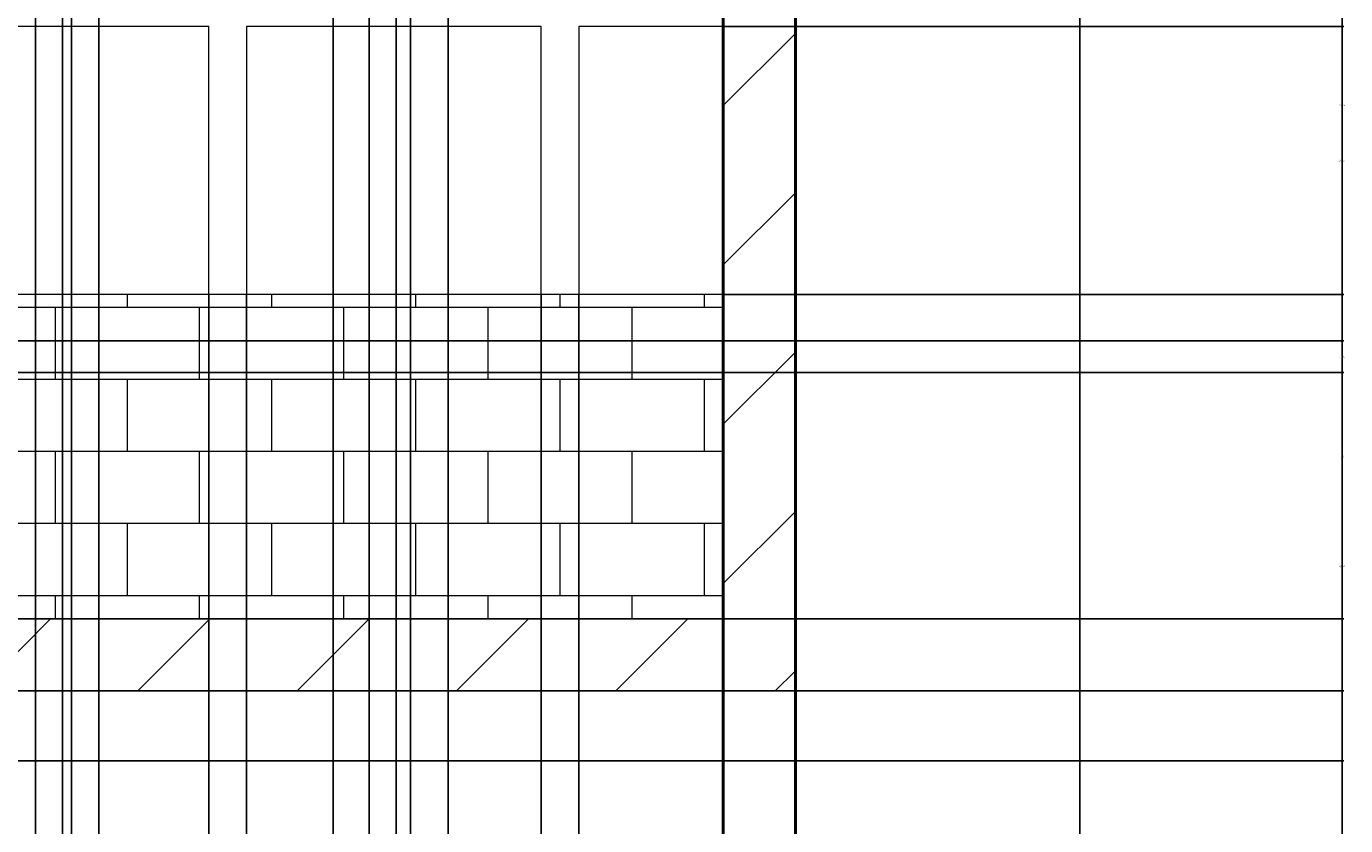
# Model space of a CAD drawing. Units: inches. Extents: x -14 to 375, y -86 to 549.
# Tile 9 of 12: x 228 to 375, y 248 to 336. Entities that reach past the tile are written whole.
import ezdxf

# ---------------------------------------------------------------- set-up
doc = ezdxf.new("R2010")
doc.units = ezdxf.units.IN
doc.header["$MEASUREMENT"] = 0
for name, color, linetype, lineweight in [('A-ANNO-DIMS', 2, 'Continuous', 18), ('A-ELEV', 7, 'Continuous', 25), ('A-ELEV-PATT', 8, 'Continuous', 13), ('A-ELEV-RAIL', 8, 'Continuous', 18)]:
    doc.layers.add(name, color=color, linetype=linetype, lineweight=lineweight)
doc.styles.get("Standard").update_dxf_attribs({"font": 'arial.ttf'})
doc.dimstyles.get("Standard").update_dxf_attribs({"dimtxt": 0.18, "dimasz": 0.18, "dimexe": 0.18, "dimexo": 0.0625, "dimgap": 0.09, "dimtad": 0, "dimtih": 1, "dimtoh": 1, "dimdec": 4, "dimzin": 0, "dimdsep": 46, "dimtxsty": 'Standard', "dimcen": 0.09, "dimadec": 0, "dimazin": 0, "dimtfac": 1, "dimtdec": 4, "dimtofl": 0, "dimtmove": 0, "dimatfit": 3, "dimfxl": 1, "dimtolj": 1, "dimtzin": 0, "dimarcsym": 0})

# ---------------------------------------------------------------- blocks, each defined once
blk = doc.blocks.new('*D10')
at = {"layer": 'A-ANNO-DIMS', "color": 0, "lineweight": -2, "transparency": 16777216}
for p, q in [((301.52, 485.96), (374.54, 485.96)), ((374.36, 485.78), (374.36, 225.61)), ((374.36, -34.93), (374.36, 225.24)), ((345.33, -35.11), (374.54, -35.11))]:
    blk.add_line(p, q, dxfattribs=at)
at = {"layer": 'A-ANNO-DIMS', "color": 0, "transparency": 16777216}
for points in [[(374.33, 485.78), (374.39, 485.78), (374.36, 485.96)], [(374.33, -34.93), (374.39, -34.93), (374.36, -35.11)]]:
    blk.add_solid(points, dxfattribs=at)
at = {"layer": 'Defpoints', "color": 0, "transparency": 16777216}
for p in [(301.46, 485.96), (374.36, 485.96), (345.26, -35.11)]:
    blk.add_point(p, dxfattribs=at)
at = {"layer": 'A-ANNO-DIMS', "color": 0, "transparency": 16777216, "insert": (374.36, 225.42), "char_height": 0.18, "attachment_point": 5}
blk.add_mtext('\\A1;521.1', dxfattribs=at)
blk = doc.blocks.new('*D33')
at = {"layer": 'A-ANNO-DIMS', "color": 0, "lineweight": -2, "transparency": 16777216}
for p, q in [((107.76, 254.96), (374.54, 254.96)), ((374.36, 254.78), (374.36, 250.64)), ((374.36, 246.14), (374.36, 250.28)), ((107.76, 245.96), (374.54, 245.96))]:
    blk.add_line(p, q, dxfattribs=at)
at = {"layer": 'A-ANNO-DIMS', "color": 0, "transparency": 16777216}
for points in [[(374.33, 254.78), (374.39, 254.78), (374.36, 254.96)], [(374.33, 246.14), (374.39, 246.14), (374.36, 245.96)]]:
    blk.add_solid(points, dxfattribs=at)
at = {"layer": 'Defpoints', "color": 0, "transparency": 16777216}
for p in [(107.7, 254.96), (374.36, 254.96), (107.7, 245.96)]:
    blk.add_point(p, dxfattribs=at)
at = {"layer": 'A-ANNO-DIMS', "color": 0, "transparency": 16777216, "insert": (374.36, 250.46), "char_height": 0.18, "attachment_point": 5}
blk.add_mtext('\\A1;9', dxfattribs=at)
blk = doc.blocks.new('*D34')
at = {"layer": 'A-ANNO-DIMS', "color": 0, "lineweight": -2, "transparency": 16777216}
for p, q in [((107.64, 298.04), (374.54, 298.04)), ((374.36, 297.86), (374.36, 276.68)), ((374.36, 255.14), (374.36, 276.32)), ((107.76, 254.96), (374.54, 254.96))]:
    blk.add_line(p, q, dxfattribs=at)
at = {"layer": 'A-ANNO-DIMS', "color": 0, "transparency": 16777216}
for points in [[(374.33, 297.86), (374.39, 297.86), (374.36, 298.04)], [(374.33, 255.14), (374.39, 255.14), (374.36, 254.96)]]:
    blk.add_solid(points, dxfattribs=at)
at = {"layer": 'Defpoints', "color": 0, "transparency": 16777216}
for p in [(107.58, 298.04), (374.36, 298.04), (107.7, 254.96)]:
    blk.add_point(p, dxfattribs=at)
at = {"layer": 'A-ANNO-DIMS', "color": 0, "transparency": 16777216, "insert": (374.36, 276.5), "char_height": 0.18, "attachment_point": 5}
blk.add_mtext('\\A1;43.08', dxfattribs=at)
blk = doc.blocks.new('*D35')
at = {"layer": 'A-ANNO-DIMS', "color": 0, "lineweight": -2, "transparency": 16777216}
for p, q in [((107.64, 301.54), (374.54, 301.54)), ((374.36, 301.36), (374.36, 299.97)), ((374.36, 298.22), (374.36, 299.6)), ((107.64, 298.04), (374.54, 298.04))]:
    blk.add_line(p, q, dxfattribs=at)
at = {"layer": 'A-ANNO-DIMS', "color": 0, "transparency": 16777216}
for points in [[(374.33, 301.36), (374.39, 301.36), (374.36, 301.54)], [(374.33, 298.22), (374.39, 298.22), (374.36, 298.04)]]:
    blk.add_solid(points, dxfattribs=at)
at = {"layer": 'Defpoints', "color": 0, "transparency": 16777216}
for p in [(107.58, 301.54), (374.36, 301.54), (107.58, 298.04)]:
    blk.add_point(p, dxfattribs=at)
at = {"layer": 'A-ANNO-DIMS', "color": 0, "transparency": 16777216, "insert": (374.36, 299.79), "char_height": 0.18, "attachment_point": 5}
blk.add_mtext('\\A1;3.501', dxfattribs=at)
blk = doc.blocks.new('*D36')
at = {"layer": 'A-ANNO-DIMS', "color": 0, "lineweight": -2, "transparency": 16777216}
for p, q in [((107.56, 353.96), (374.54, 353.96)), ((374.36, 353.78), (374.36, 327.93)), ((374.36, 301.72), (374.36, 327.57)), ((107.64, 301.54), (374.54, 301.54))]:
    blk.add_line(p, q, dxfattribs=at)
at = {"layer": 'A-ANNO-DIMS', "color": 0, "transparency": 16777216}
for points in [[(374.33, 353.78), (374.39, 353.78), (374.36, 353.96)], [(374.33, 301.72), (374.39, 301.72), (374.36, 301.54)]]:
    blk.add_solid(points, dxfattribs=at)
at = {"layer": 'Defpoints', "color": 0, "transparency": 16777216}
for p in [(107.5, 353.96), (374.36, 353.96), (107.58, 301.54)]:
    blk.add_point(p, dxfattribs=at)
at = {"layer": 'A-ANNO-DIMS', "color": 0, "transparency": 16777216, "insert": (374.36, 327.75), "char_height": 0.18, "attachment_point": 5}
blk.add_mtext('\\A1;52.42', dxfattribs=at)
blk = doc.blocks.new('*D43')
at = {"layer": 'A-ANNO-DIMS', "color": 0, "lineweight": -2, "transparency": 16777216}
for p, q in [((142.23, 270.64), (142.23, -64.39)), ((305.63, 270.64), (305.63, -64.39)), ((142.41, -64.21), (223.55, -64.21)), ((305.45, -64.21), (224.32, -64.21))]:
    blk.add_line(p, q, dxfattribs=at)
at = {"layer": 'A-ANNO-DIMS', "color": 0, "transparency": 16777216}
for points in [[(142.41, -64.18), (142.41, -64.24), (142.23, -64.21)], [(305.45, -64.18), (305.45, -64.24), (305.63, -64.21)]]:
    blk.add_solid(points, dxfattribs=at)
at = {"layer": 'Defpoints', "color": 0, "transparency": 16777216}
for p in [(142.23, 270.71), (305.63, 270.71), (305.63, -64.21)]:
    blk.add_point(p, dxfattribs=at)
at = {"layer": 'A-ANNO-DIMS', "color": 0, "transparency": 16777216, "insert": (223.93, -64.21), "char_height": 0.18, "attachment_point": 5}
blk.add_mtext('\\A1;163.4', dxfattribs=at)
blk = doc.blocks.new('*D44')
at = {"layer": 'A-ANNO-DIMS', "color": 0, "lineweight": -2, "transparency": 16777216}
for p, q in [((305.63, 270.64), (305.63, -64.39)), ((313.63, 262.64), (313.63, -64.39)), ((305.81, -64.21), (309.48, -64.21)), ((313.45, -64.21), (309.78, -64.21))]:
    blk.add_line(p, q, dxfattribs=at)
at = {"layer": 'A-ANNO-DIMS', "color": 0, "transparency": 16777216}
for points in [[(305.81, -64.18), (305.81, -64.24), (305.63, -64.21)], [(313.45, -64.18), (313.45, -64.24), (313.63, -64.21)]]:
    blk.add_solid(points, dxfattribs=at)
at = {"layer": 'Defpoints', "color": 0, "transparency": 16777216}
for p in [(305.63, 270.71), (313.63, 262.71), (313.63, -64.21)]:
    blk.add_point(p, dxfattribs=at)
at = {"layer": 'A-ANNO-DIMS', "color": 0, "transparency": 16777216, "insert": (309.63, -64.21), "char_height": 0.18, "attachment_point": 5}
blk.add_mtext('\\A1;8', dxfattribs=at)
blk = doc.blocks.new('*D49')
at = {"layer": 'A-ANNO-DIMS', "color": 0, "lineweight": -2, "transparency": 16777216}
for p, q in [((215.95, 306.64), (215.95, -64.39)), ((248.64, 306.64), (248.64, -64.39)), ((216.13, -64.21), (231.9, -64.21)), ((248.46, -64.21), (232.69, -64.21))]:
    blk.add_line(p, q, dxfattribs=at)
at = {"layer": 'A-ANNO-DIMS', "color": 0, "transparency": 16777216}
for points in [[(216.13, -64.18), (216.13, -64.24), (215.95, -64.21)], [(248.46, -64.18), (248.46, -64.24), (248.64, -64.21)]]:
    blk.add_solid(points, dxfattribs=at)
at = {"layer": 'Defpoints', "color": 0, "transparency": 16777216}
for p in [(215.95, 306.71), (248.64, 306.71), (248.64, -64.21)]:
    blk.add_point(p, dxfattribs=at)
at = {"layer": 'A-ANNO-DIMS', "color": 0, "transparency": 16777216, "insert": (232.29, -64.21), "char_height": 0.18, "attachment_point": 5}
blk.add_mtext('\\A1;32.69', dxfattribs=at)
blk = doc.blocks.new('*D50')
at = {"layer": 'A-ANNO-DIMS', "color": 0, "lineweight": -2, "transparency": 16777216}
for p, q in [((248.64, 306.64), (248.64, -64.39)), ((252.81, 306.64), (252.81, -64.39)), ((248.82, -64.21), (250.39, -64.21)), ((252.63, -64.21), (251.05, -64.21))]:
    blk.add_line(p, q, dxfattribs=at)
at = {"layer": 'A-ANNO-DIMS', "color": 0, "transparency": 16777216}
for points in [[(248.82, -64.18), (248.82, -64.24), (248.64, -64.21)], [(252.63, -64.18), (252.63, -64.24), (252.81, -64.21)]]:
    blk.add_solid(points, dxfattribs=at)
at = {"layer": 'Defpoints', "color": 0, "transparency": 16777216}
for p in [(248.64, 306.71), (252.81, 306.71), (252.81, -64.21)]:
    blk.add_point(p, dxfattribs=at)
at = {"layer": 'A-ANNO-DIMS', "color": 0, "transparency": 16777216, "insert": (250.72, -64.21), "char_height": 0.18, "attachment_point": 5}
blk.add_mtext('\\A1;4.17', dxfattribs=at)
blk = doc.blocks.new('*D51')
at = {"layer": 'A-ANNO-DIMS', "color": 0, "lineweight": -2, "transparency": 16777216}
for p, q in [((252.81, 306.64), (252.81, -64.39)), ((285.5, 306.64), (285.5, -64.39)), ((252.99, -64.21), (268.76, -64.21)), ((285.32, -64.21), (269.54, -64.21))]:
    blk.add_line(p, q, dxfattribs=at)
at = {"layer": 'A-ANNO-DIMS', "color": 0, "transparency": 16777216}
for points in [[(252.99, -64.18), (252.99, -64.24), (252.81, -64.21)], [(285.32, -64.18), (285.32, -64.24), (285.5, -64.21)]]:
    blk.add_solid(points, dxfattribs=at)
at = {"layer": 'Defpoints', "color": 0, "transparency": 16777216}
for p in [(252.81, 306.71), (285.5, 306.71), (285.5, -64.21)]:
    blk.add_point(p, dxfattribs=at)
at = {"layer": 'A-ANNO-DIMS', "color": 0, "transparency": 16777216, "insert": (269.15, -64.21), "char_height": 0.18, "attachment_point": 5}
blk.add_mtext('\\A1;32.69', dxfattribs=at)
blk = doc.blocks.new('*D52')
at = {"layer": 'A-ANNO-DIMS', "color": 0, "lineweight": -2, "transparency": 16777216}
for p, q in [((285.5, 306.64), (285.5, -64.39)), ((289.66, 306.64), (289.66, -64.39)), ((285.68, -64.21), (287.25, -64.21)), ((289.48, -64.21), (287.91, -64.21))]:
    blk.add_line(p, q, dxfattribs=at)
at = {"layer": 'A-ANNO-DIMS', "color": 0, "transparency": 16777216}
for points in [[(285.68, -64.18), (285.68, -64.24), (285.5, -64.21)], [(289.48, -64.18), (289.48, -64.24), (289.66, -64.21)]]:
    blk.add_solid(points, dxfattribs=at)
at = {"layer": 'Defpoints', "color": 0, "transparency": 16777216}
for p in [(285.5, 306.71), (289.66, 306.71), (289.66, -64.21)]:
    blk.add_point(p, dxfattribs=at)
at = {"layer": 'A-ANNO-DIMS', "color": 0, "transparency": 16777216, "insert": (287.58, -64.21), "char_height": 0.18, "attachment_point": 5}
blk.add_mtext('\\A1;4.17', dxfattribs=at)
blk = doc.blocks.new('*D57')
at = {"layer": 'A-ANNO-DIMS', "color": 0, "lineweight": -2, "transparency": 16777216}
for p, q in [((229.41, 340.38), (229.41, -64.39)), ((232.41, 340.38), (232.41, -64.39)), ((229.59, -64.21), (230.76, -64.21)), ((232.23, -64.21), (231.06, -64.21))]:
    blk.add_line(p, q, dxfattribs=at)
at = {"layer": 'A-ANNO-DIMS', "color": 0, "transparency": 16777216}
for points in [[(229.59, -64.18), (229.59, -64.24), (229.41, -64.21)], [(232.23, -64.18), (232.23, -64.24), (232.41, -64.21)]]:
    blk.add_solid(points, dxfattribs=at)
at = {"layer": 'Defpoints', "color": 0, "transparency": 16777216}
for p in [(229.41, 340.44), (232.41, 340.44), (232.41, -64.21)]:
    blk.add_point(p, dxfattribs=at)
at = {"layer": 'A-ANNO-DIMS', "color": 0, "transparency": 16777216, "insert": (230.91, -64.21), "char_height": 0.18, "attachment_point": 5}
blk.add_mtext('\\A1;3', dxfattribs=at)
blk = doc.blocks.new('*D58')
at = {"layer": 'A-ANNO-DIMS', "color": 0, "lineweight": -2, "transparency": 16777216}
for p, q in [((232.41, 340.38), (232.41, -64.39)), ((236.41, 340.38), (236.41, -64.39)), ((232.59, -64.21), (234.26, -64.21)), ((236.23, -64.21), (234.56, -64.21))]:
    blk.add_line(p, q, dxfattribs=at)
at = {"layer": 'A-ANNO-DIMS', "color": 0, "transparency": 16777216}
for points in [[(232.59, -64.18), (232.59, -64.24), (232.41, -64.21)], [(236.23, -64.18), (236.23, -64.24), (236.41, -64.21)]]:
    blk.add_solid(points, dxfattribs=at)
at = {"layer": 'Defpoints', "color": 0, "transparency": 16777216}
for p in [(232.41, 340.44), (236.41, 340.44), (236.41, -64.21)]:
    blk.add_point(p, dxfattribs=at)
at = {"layer": 'A-ANNO-DIMS', "color": 0, "transparency": 16777216, "insert": (234.41, -64.21), "char_height": 0.18, "attachment_point": 5}
blk.add_mtext('\\A1;4', dxfattribs=at)
blk = doc.blocks.new('*D59')
at = {"layer": 'A-ANNO-DIMS', "color": 0, "lineweight": -2, "transparency": 16777216}
for p, q in [((236.41, 340.38), (236.41, -64.39)), ((262.41, 340.38), (262.41, -64.39)), ((236.59, -64.21), (249.19, -64.21)), ((262.23, -64.21), (249.63, -64.21))]:
    blk.add_line(p, q, dxfattribs=at)
at = {"layer": 'A-ANNO-DIMS', "color": 0, "transparency": 16777216}
for points in [[(236.59, -64.18), (236.59, -64.24), (236.41, -64.21)], [(262.23, -64.18), (262.23, -64.24), (262.41, -64.21)]]:
    blk.add_solid(points, dxfattribs=at)
at = {"layer": 'Defpoints', "color": 0, "transparency": 16777216}
for p in [(236.41, 340.44), (262.41, 340.44), (262.41, -64.21)]:
    blk.add_point(p, dxfattribs=at)
at = {"layer": 'A-ANNO-DIMS', "color": 0, "transparency": 16777216, "insert": (249.41, -64.21), "char_height": 0.18, "attachment_point": 5}
blk.add_mtext('\\A1;26', dxfattribs=at)
blk = doc.blocks.new('*D60')
at = {"layer": 'A-ANNO-DIMS', "color": 0, "lineweight": -2, "transparency": 16777216}
for p, q in [((262.41, 340.38), (262.41, -64.39)), ((266.41, 340.38), (266.41, -64.39)), ((262.59, -64.21), (264.26, -64.21)), ((266.23, -64.21), (264.56, -64.21))]:
    blk.add_line(p, q, dxfattribs=at)
at = {"layer": 'A-ANNO-DIMS', "color": 0, "transparency": 16777216}
for points in [[(262.59, -64.18), (262.59, -64.24), (262.41, -64.21)], [(266.23, -64.18), (266.23, -64.24), (266.41, -64.21)]]:
    blk.add_solid(points, dxfattribs=at)
at = {"layer": 'Defpoints', "color": 0, "transparency": 16777216}
for p in [(262.41, 340.44), (266.41, 340.44), (266.41, -64.21)]:
    blk.add_point(p, dxfattribs=at)
at = {"layer": 'A-ANNO-DIMS', "color": 0, "transparency": 16777216, "insert": (264.41, -64.21), "char_height": 0.18, "attachment_point": 5}
blk.add_mtext('\\A1;4', dxfattribs=at)
blk = doc.blocks.new('*D61')
at = {"layer": 'A-ANNO-DIMS', "color": 0, "lineweight": -2, "transparency": 16777216}
for p, q in [((266.41, 340.38), (266.41, -64.39)), ((269.41, 340.38), (269.41, -64.39)), ((266.59, -64.21), (267.76, -64.21)), ((269.23, -64.21), (268.06, -64.21))]:
    blk.add_line(p, q, dxfattribs=at)
at = {"layer": 'A-ANNO-DIMS', "color": 0, "transparency": 16777216}
for points in [[(266.59, -64.18), (266.59, -64.24), (266.41, -64.21)], [(269.23, -64.18), (269.23, -64.24), (269.41, -64.21)]]:
    blk.add_solid(points, dxfattribs=at)
at = {"layer": 'Defpoints', "color": 0, "transparency": 16777216}
for p in [(266.41, 340.44), (269.41, 340.44), (269.41, -64.21)]:
    blk.add_point(p, dxfattribs=at)
at = {"layer": 'A-ANNO-DIMS', "color": 0, "transparency": 16777216, "insert": (267.91, -64.21), "char_height": 0.18, "attachment_point": 5}
blk.add_mtext('\\A1;3', dxfattribs=at)
blk = doc.blocks.new('*D62')
at = {"layer": 'A-ANNO-DIMS', "color": 0, "lineweight": -2, "transparency": 16777216}
for p, q in [((305.69, 270.71), (374.54, 270.71)), ((374.36, 270.53), (374.36, 266.89)), ((374.36, 262.89), (374.36, 266.53)), ((313.69, 262.71), (374.54, 262.71))]:
    blk.add_line(p, q, dxfattribs=at)
at = {"layer": 'A-ANNO-DIMS', "color": 0, "transparency": 16777216}
for points in [[(374.33, 270.53), (374.39, 270.53), (374.36, 270.71)], [(374.33, 262.89), (374.39, 262.89), (374.36, 262.71)]]:
    blk.add_solid(points, dxfattribs=at)
at = {"layer": 'Defpoints', "color": 0, "transparency": 16777216}
for p in [(305.63, 270.71), (374.36, 270.71), (313.63, 262.71)]:
    blk.add_point(p, dxfattribs=at)
at = {"layer": 'A-ANNO-DIMS', "color": 0, "transparency": 16777216, "insert": (374.36, 266.71), "char_height": 0.18, "attachment_point": 5}
blk.add_mtext('\\A1;8', dxfattribs=at)
blk = doc.blocks.new('*D63')
at = {"layer": 'A-ANNO-DIMS', "color": 0, "lineweight": -2, "transparency": 16777216}
for p, q in [((305.69, 306.71), (374.54, 306.71)), ((374.36, 306.53), (374.36, 288.89)), ((374.36, 270.89), (374.36, 288.53)), ((305.69, 270.71), (374.54, 270.71))]:
    blk.add_line(p, q, dxfattribs=at)
at = {"layer": 'A-ANNO-DIMS', "color": 0, "transparency": 16777216}
for points in [[(374.33, 306.53), (374.39, 306.53), (374.36, 306.71)], [(374.33, 270.89), (374.39, 270.89), (374.36, 270.71)]]:
    blk.add_solid(points, dxfattribs=at)
at = {"layer": 'Defpoints', "color": 0, "transparency": 16777216}
for p in [(305.63, 306.71), (374.36, 306.71), (305.63, 270.71)]:
    blk.add_point(p, dxfattribs=at)
at = {"layer": 'A-ANNO-DIMS', "color": 0, "transparency": 16777216, "insert": (374.36, 288.71), "char_height": 0.18, "attachment_point": 5}
blk.add_mtext('\\A1;36', dxfattribs=at)
blk = doc.blocks.new('*D64')
at = {"layer": 'A-ANNO-DIMS', "color": 0, "lineweight": -2, "transparency": 16777216}
for p, q in [((305.69, 336.44), (374.54, 336.44)), ((374.36, 336.26), (374.36, 321.76)), ((374.36, 306.89), (374.36, 321.39)), ((305.69, 306.71), (374.54, 306.71))]:
    blk.add_line(p, q, dxfattribs=at)
at = {"layer": 'A-ANNO-DIMS', "color": 0, "transparency": 16777216}
for points in [[(374.33, 336.26), (374.39, 336.26), (374.36, 336.44)], [(374.33, 306.89), (374.39, 306.89), (374.36, 306.71)]]:
    blk.add_solid(points, dxfattribs=at)
at = {"layer": 'Defpoints', "color": 0, "transparency": 16777216}
for p in [(305.63, 336.44), (374.36, 336.44), (305.63, 306.71)]:
    blk.add_point(p, dxfattribs=at)
at = {"layer": 'A-ANNO-DIMS', "color": 0, "transparency": 16777216, "insert": (374.36, 321.57), "char_height": 0.18, "attachment_point": 5}
blk.add_mtext('\\A1;29.735', dxfattribs=at)
blk = doc.blocks.new('*D72')
at = {"layer": 'A-ANNO-DIMS', "color": 0, "lineweight": -2, "transparency": 16777216}
for p, q in [((229.41, 126.03), (229.41, 515.24)), ((233.41, 168.03), (233.41, 515.24)), ((229.59, 515.06), (231.26, 515.06)), ((233.23, 515.06), (231.56, 515.06))]:
    blk.add_line(p, q, dxfattribs=at)
at = {"layer": 'A-ANNO-DIMS', "color": 0, "transparency": 16777216}
for points in [[(229.59, 515.09), (229.59, 515.03), (229.41, 515.06)], [(233.23, 515.09), (233.23, 515.03), (233.41, 515.06)]]:
    blk.add_solid(points, dxfattribs=at)
at = {"layer": 'Defpoints', "color": 0, "transparency": 16777216}
for p in [(233.41, 515.06), (233.41, 167.97), (229.41, 125.97)]:
    blk.add_point(p, dxfattribs=at)
at = {"layer": 'A-ANNO-DIMS', "color": 0, "transparency": 16777216, "insert": (231.41, 515.06), "char_height": 0.18, "attachment_point": 5}
blk.add_mtext('\\A1;4', dxfattribs=at)
blk = doc.blocks.new('*D85')
at = {"layer": 'A-ANNO-DIMS', "color": 0, "lineweight": -2, "transparency": 16777216}
for p, q in [((229.41, 210.03), (229.41, 515.24)), ((232.41, 207.01), (232.41, 515.24)), ((229.59, 515.06), (230.76, 515.06)), ((232.23, 515.06), (231.06, 515.06))]:
    blk.add_line(p, q, dxfattribs=at)
at = {"layer": 'A-ANNO-DIMS', "color": 0, "transparency": 16777216}
for points in [[(229.59, 515.09), (229.59, 515.03), (229.41, 515.06)], [(232.23, 515.09), (232.23, 515.03), (232.41, 515.06)]]:
    blk.add_solid(points, dxfattribs=at)
at = {"layer": 'Defpoints', "color": 0, "transparency": 16777216}
for p in [(232.41, 515.06), (229.41, 209.97), (232.41, 206.95)]:
    blk.add_point(p, dxfattribs=at)
at = {"layer": 'A-ANNO-DIMS', "color": 0, "transparency": 16777216, "insert": (230.91, 515.06), "char_height": 0.18, "attachment_point": 5}
blk.add_mtext('\\A1;3', dxfattribs=at)
blk = doc.blocks.new('*D86')
at = {"layer": 'A-ANNO-DIMS', "color": 0, "lineweight": -2, "transparency": 16777216}
for p, q in [((232.41, 207.01), (232.41, 515.24)), ((236.41, 201.01), (236.41, 515.24)), ((232.59, 515.06), (234.26, 515.06)), ((236.23, 515.06), (234.56, 515.06))]:
    blk.add_line(p, q, dxfattribs=at)
at = {"layer": 'A-ANNO-DIMS', "color": 0, "transparency": 16777216}
for points in [[(232.59, 515.09), (232.59, 515.03), (232.41, 515.06)], [(236.23, 515.09), (236.23, 515.03), (236.41, 515.06)]]:
    blk.add_solid(points, dxfattribs=at)
at = {"layer": 'Defpoints', "color": 0, "transparency": 16777216}
for p in [(236.41, 515.06), (232.41, 206.95), (236.41, 200.95)]:
    blk.add_point(p, dxfattribs=at)
at = {"layer": 'A-ANNO-DIMS', "color": 0, "transparency": 16777216, "insert": (234.41, 515.06), "char_height": 0.18, "attachment_point": 5}
blk.add_mtext('\\A1;4', dxfattribs=at)
blk = doc.blocks.new('*D87')
at = {"layer": 'A-ANNO-DIMS', "color": 0, "lineweight": -2, "transparency": 16777216}
for p, q in [((236.41, 201.01), (236.41, 515.24)), ((262.41, 201.01), (262.41, 515.24)), ((236.59, 515.06), (249.19, 515.06)), ((262.23, 515.06), (249.63, 515.06))]:
    blk.add_line(p, q, dxfattribs=at)
at = {"layer": 'A-ANNO-DIMS', "color": 0, "transparency": 16777216}
for points in [[(236.59, 515.09), (236.59, 515.03), (236.41, 515.06)], [(262.23, 515.09), (262.23, 515.03), (262.41, 515.06)]]:
    blk.add_solid(points, dxfattribs=at)
at = {"layer": 'Defpoints', "color": 0, "transparency": 16777216}
for p in [(262.41, 515.06), (236.41, 200.95), (262.41, 200.95)]:
    blk.add_point(p, dxfattribs=at)
at = {"layer": 'A-ANNO-DIMS', "color": 0, "transparency": 16777216, "insert": (249.41, 515.06), "char_height": 0.18, "attachment_point": 5}
blk.add_mtext('\\A1;26', dxfattribs=at)
blk = doc.blocks.new('*D88')
at = {"layer": 'A-ANNO-DIMS', "color": 0, "lineweight": -2, "transparency": 16777216}
for p, q in [((262.41, 201.01), (262.41, 515.24)), ((266.41, 207.01), (266.41, 515.24)), ((262.59, 515.06), (264.26, 515.06)), ((266.23, 515.06), (264.56, 515.06))]:
    blk.add_line(p, q, dxfattribs=at)
at = {"layer": 'A-ANNO-DIMS', "color": 0, "transparency": 16777216}
for points in [[(262.59, 515.09), (262.59, 515.03), (262.41, 515.06)], [(266.23, 515.09), (266.23, 515.03), (266.41, 515.06)]]:
    blk.add_solid(points, dxfattribs=at)
at = {"layer": 'Defpoints', "color": 0, "transparency": 16777216}
for p in [(266.41, 515.06), (266.41, 206.95), (262.41, 200.95)]:
    blk.add_point(p, dxfattribs=at)
at = {"layer": 'A-ANNO-DIMS', "color": 0, "transparency": 16777216, "insert": (264.41, 515.06), "char_height": 0.18, "attachment_point": 5}
blk.add_mtext('\\A1;4', dxfattribs=at)
blk = doc.blocks.new('*D89')
at = {"layer": 'A-ANNO-DIMS', "color": 0, "lineweight": -2, "transparency": 16777216}
for p, q in [((266.41, 207.01), (266.41, 515.24)), ((269.41, 210.03), (269.41, 515.24)), ((266.59, 515.06), (267.76, 515.06)), ((269.23, 515.06), (268.06, 515.06))]:
    blk.add_line(p, q, dxfattribs=at)
at = {"layer": 'A-ANNO-DIMS', "color": 0, "transparency": 16777216}
for points in [[(266.59, 515.09), (266.59, 515.03), (266.41, 515.06)], [(269.23, 515.09), (269.23, 515.03), (269.41, 515.06)]]:
    blk.add_solid(points, dxfattribs=at)
at = {"layer": 'Defpoints', "color": 0, "transparency": 16777216}
for p in [(269.41, 515.06), (269.41, 209.97), (266.41, 206.95)]:
    blk.add_point(p, dxfattribs=at)
at = {"layer": 'A-ANNO-DIMS', "color": 0, "transparency": 16777216, "insert": (267.91, 515.06), "char_height": 0.18, "attachment_point": 5}
blk.add_mtext('\\A1;3', dxfattribs=at)
blk = doc.blocks.new('*D104')
at = {"layer": 'A-ANNO-DIMS', "color": 0, "lineweight": -2, "transparency": 16777216}
for p, q in [((190.15, 6.02), (190.15, 515.24)), ((271, 6.02), (271, 515.24)), ((190.33, 515.06), (230.18, 515.06)), ((270.82, 515.06), (230.97, 515.06))]:
    blk.add_line(p, q, dxfattribs=at)
at = {"layer": 'A-ANNO-DIMS', "color": 0, "transparency": 16777216}
for points in [[(190.33, 515.09), (190.33, 515.03), (190.15, 515.06)], [(270.82, 515.09), (270.82, 515.03), (271, 515.06)]]:
    blk.add_solid(points, dxfattribs=at)
at = {"layer": 'Defpoints', "color": 0, "transparency": 16777216}
for p in [(271, 515.06), (190.15, 5.96), (271, 5.96)]:
    blk.add_point(p, dxfattribs=at)
at = {"layer": 'A-ANNO-DIMS', "color": 0, "transparency": 16777216, "insert": (230.57, 515.06), "char_height": 0.18, "attachment_point": 5}
blk.add_mtext('\\A1;80.85', dxfattribs=at)
blk = doc.blocks.new('*D105')
at = {"layer": 'A-ANNO-DIMS', "color": 0, "lineweight": -2, "transparency": 16777216}
for p, q in [((271, 6.02), (271, 515.24)), ((275.19, 6.02), (275.19, 515.24)), ((271.18, 515.06), (272.69, 515.06)), ((275.01, 515.06), (273.49, 515.06))]:
    blk.add_line(p, q, dxfattribs=at)
at = {"layer": 'A-ANNO-DIMS', "color": 0, "transparency": 16777216}
for points in [[(271.18, 515.09), (271.18, 515.03), (271, 515.06)], [(275.01, 515.09), (275.01, 515.03), (275.19, 515.06)]]:
    blk.add_solid(points, dxfattribs=at)
at = {"layer": 'Defpoints', "color": 0, "transparency": 16777216}
for p in [(275.19, 515.06), (271, 5.96), (275.19, 5.96)]:
    blk.add_point(p, dxfattribs=at)
at = {"layer": 'A-ANNO-DIMS', "color": 0, "transparency": 16777216, "insert": (273.09, 515.06), "char_height": 0.18, "attachment_point": 5}
blk.add_mtext('\\A1;4.186', dxfattribs=at)
blk = doc.blocks.new('*D106')
at = {"layer": 'A-ANNO-DIMS', "color": 0, "lineweight": -2, "transparency": 16777216}
for p, q in [((275.19, 6.02), (275.19, 515.24)), ((305.77, 6.02), (305.77, 515.24)), ((275.37, 515.06), (290.01, 515.06)), ((305.59, 515.06), (290.94, 515.06))]:
    blk.add_line(p, q, dxfattribs=at)
at = {"layer": 'A-ANNO-DIMS', "color": 0, "transparency": 16777216}
for points in [[(275.37, 515.09), (275.37, 515.03), (275.19, 515.06)], [(305.59, 515.09), (305.59, 515.03), (305.77, 515.06)]]:
    blk.add_solid(points, dxfattribs=at)
at = {"layer": 'Defpoints', "color": 0, "transparency": 16777216}
for p in [(305.77, 515.06), (275.19, 5.96), (305.77, 5.96)]:
    blk.add_point(p, dxfattribs=at)
at = {"layer": 'A-ANNO-DIMS', "color": 0, "transparency": 16777216, "insert": (290.48, 515.06), "char_height": 0.18, "attachment_point": 5}
blk.add_mtext('\\A1;30.585', dxfattribs=at)
blk = doc.blocks.new('*D107')
at = {"layer": 'A-ANNO-DIMS', "color": 0, "lineweight": -2, "transparency": 16777216}
for p, q in [((305.77, 6.02), (305.77, 515.24)), ((313.77, 6.02), (313.77, 515.24)), ((305.95, 515.06), (309.62, 515.06)), ((313.59, 515.06), (309.92, 515.06))]:
    blk.add_line(p, q, dxfattribs=at)
at = {"layer": 'A-ANNO-DIMS', "color": 0, "transparency": 16777216}
for points in [[(305.95, 515.09), (305.95, 515.03), (305.77, 515.06)], [(313.59, 515.09), (313.59, 515.03), (313.77, 515.06)]]:
    blk.add_solid(points, dxfattribs=at)
at = {"layer": 'Defpoints', "color": 0, "transparency": 16777216}
for p in [(313.77, 515.06), (305.77, 5.96), (313.77, 5.96)]:
    blk.add_point(p, dxfattribs=at)
at = {"layer": 'A-ANNO-DIMS', "color": 0, "transparency": 16777216, "insert": (309.77, 515.06), "char_height": 0.18, "attachment_point": 5}
blk.add_mtext('\\A1;8', dxfattribs=at)

msp = doc.modelspace()

# ---------------------------------------------------------------- hatches: boundary and pattern name
at = {"layer": 'A-ELEV-PATT'}
h = msp.add_hatch(dxfattribs=at)
h.set_pattern_fill('ANSI31', color=256, scale=100)
h.set_pattern_definition([(45, (-168.406, -22.703), (-8.83883, 8.83883), [])])
h.paths.add_polyline_path([(313.6281, 262.7071), (313.6281, 357.9589), (313.7701, 357.9589), (313.7701, 433.1717, 0.36940998), (134.2334, 433.1717), (134.2334, 365.9589), (134.2334, 262.7071)])
h.paths.add_polyline_path([(142.2334, 270.7071), (142.2334, 365.9589), (142.2334, 429.4208, -0.35358711), (305.7701, 429.4208), (305.7701, 365.9589), (305.6281, 365.9589), (305.6281, 270.7071)], flags=16)
h.paths.add_polyline_path([(134.2334, 187.8466), (134.2334, 117.9589), (313.7701, 117.9589), (313.7701, 187.8466, 0.62486768)])
h.paths.add_polyline_path([(305.7701, 185.9589), (305.7701, 125.9589), (142.2334, 125.9589), (142.2334, 185.9589, -0.61125102)], flags=16)
h.paths.add_polyline_path([(134.2334, 73.1717), (134.2334, 5.9589), (142.2334, 5.9589), (142.2334, 69.4208, -0.35358711), (305.7701, 69.4208), (305.7701, 5.9589), (313.7701, 5.9589), (313.7701, 73.1717, 0.36940998)])
h = msp.add_hatch(dxfattribs=at)
h.set_pattern_fill('AR-B816', color=256)
h.set_pattern_definition([(0, (-168.406, -22.703), (0, 8), []), (90, (-168.406, -22.703), (-8, 8), [8, -8])])
h.paths.add_polyline_path([(305.6281, 306.7071), (142.2334, 306.7071), (142.2334, 270.7071), (305.6281, 270.7071)])

# ---------------------------------------------------------------- linework, layer by layer
at = {"layer": 'A-ELEV'}
msp.add_lwpolyline([(345.2647, 5.9589), (345.2647, 125.9589), (345.2647, 245.9589), (345.2647, 365.9589), (345.2647, 442.1495, 0.41421356), (301.4553, 485.9589)], format="xyb", dxfattribs=at)
for points in [[(134.2334, 262.7071), (313.6281, 262.7071), (313.6281, 357.9589), (313.7701, 357.9589), (313.7701, 433.1717, 0.36940998), (134.2334, 433.1717), (134.2334, 365.9589)], [(142.2334, 270.7071), (305.6281, 270.7071), (305.6281, 365.9589), (305.7701, 365.9589), (305.7701, 429.4208, 0.35358711), (142.2334, 429.4208), (142.2334, 365.9589)]]:
    msp.add_lwpolyline(points, format="xyb", close=True, dxfattribs=at)
at = {"layer": 'A-ELEV-RAIL'}
for p, q in [((248.639, 336.4421), (215.9481, 336.4421)), ((285.4964, 336.4421), (252.8055, 336.4421)), ((285.4964, 336.4421), (252.8055, 336.4421)), ((305.6281, 336.4421), (289.6628, 336.4421)), ((305.6281, 306.7071), (142.2334, 306.7071))]:
    msp.add_line(p, q, dxfattribs=at)
for points in [[(252.8055, 336.4421), (252.8055, 306.7071), (248.639, 306.7071), (248.639, 336.4421)], [(289.6628, 336.4421), (289.6628, 306.7071), (285.4964, 306.7071), (285.4964, 336.4421)]]:
    msp.add_lwpolyline(points, dxfattribs=at)

# ---------------------------------------------------------------- dimensions: what is measured, and where the dimension line sits
at = {"layer": 'A-ANNO-DIMS'}
for base, p1, p2, override, picture, middle in [((270.9993, 515.0589), (190.148, 5.9589), (270.9993, 5.9589), {"dimdec": 2, "dimlfac": 1, "dimrnd": 0, "dimzin": 0, "dimdsep": 46, "dimlunit": 2}, '*D104', (230.5736, 515.0589)), ((233.409, 515.0589), (229.409, 125.9717), (233.409, 167.9717), {"dimdec": 0, "dimlfac": 1, "dimrnd": 0, "dimzin": 0, "dimdsep": 46, "dimlunit": 2}, '*D72', (231.409, 515.0589)), ((232.409, 515.0589), (229.409, 209.9717), (232.409, 206.9487), {"dimdec": 0, "dimlfac": 1, "dimrnd": 0, "dimzin": 0, "dimdsep": 46, "dimlunit": 2}, '*D85', (230.909, 515.0589)), ((236.409, 515.0589), (232.409, 206.9487), (236.409, 200.9487), {"dimdec": 0, "dimlfac": 1, "dimrnd": 0, "dimzin": 0, "dimdsep": 46, "dimlunit": 2}, '*D86', (234.409, 515.0589)), ((262.409, 515.0589), (236.409, 200.9487), (262.409, 200.9487), {"dimdec": 0, "dimlfac": 1, "dimrnd": 0, "dimzin": 0, "dimdsep": 46, "dimlunit": 2}, '*D87', (249.409, 515.0589)), ((266.409, 515.0589), (262.409, 200.9487), (266.409, 206.9487), {"dimdec": 0, "dimlfac": 1, "dimrnd": 0, "dimzin": 0, "dimdsep": 46, "dimlunit": 2}, '*D88', (264.409, 515.0589)), ((269.409, 515.0589), (266.409, 206.9487), (269.409, 209.9717), {"dimdec": 0, "dimlfac": 1, "dimrnd": 0, "dimzin": 0, "dimdsep": 46, "dimlunit": 2}, '*D89', (267.909, 515.0589)), ((275.185, 515.0589), (270.9993, 5.9589), (275.185, 5.9589), {"dimdec": 3, "dimlfac": 1, "dimrnd": 0, "dimzin": 0, "dimdsep": 46, "dimlunit": 2}, '*D105', (273.0921, 515.0589)), ((305.7701, 515.0589), (275.185, 5.9589), (305.7701, 5.9589), {"dimdec": 3, "dimlfac": 1, "dimrnd": 0, "dimzin": 0, "dimdsep": 46, "dimlunit": 2}, '*D106', (290.4775, 515.0589)), ((313.7701, 515.0589), (305.7701, 5.9589), (313.7701, 5.9589), {"dimdec": 0, "dimlfac": 1, "dimrnd": 0, "dimzin": 0, "dimdsep": 46, "dimlunit": 2}, '*D107', (309.7701, 515.0589)), ((232.409, -64.2115), (229.409, 340.4421), (232.409, 340.4421), {"dimdec": 0, "dimlfac": 1, "dimrnd": 0, "dimzin": 0, "dimdsep": 46, "dimlunit": 2}, '*D57', (230.909, -64.2115)), ((236.409, -64.2115), (232.409, 340.4421), (236.409, 340.4421), {"dimdec": 0, "dimlfac": 1, "dimrnd": 0, "dimzin": 0, "dimdsep": 46, "dimlunit": 2}, '*D58', (234.409, -64.2115)), ((262.409, -64.2115), (236.409, 340.4421), (262.409, 340.4421), {"dimdec": 0, "dimlfac": 1, "dimrnd": 0, "dimzin": 0, "dimdsep": 46, "dimlunit": 2}, '*D59', (249.409, -64.2115)), ((266.409, -64.2115), (262.409, 340.4421), (266.409, 340.4421), {"dimdec": 0, "dimlfac": 1, "dimrnd": 0, "dimzin": 0, "dimdsep": 46, "dimlunit": 2}, '*D60', (264.409, -64.2115)), ((269.409, -64.2115), (266.409, 340.4421), (269.409, 340.4421), {"dimdec": 0, "dimlfac": 1, "dimrnd": 0, "dimzin": 0, "dimdsep": 46, "dimlunit": 2}, '*D61', (267.909, -64.2115)), ((248.639, -64.2115), (215.9481, 306.7071), (248.639, 306.7071), {"dimdec": 2, "dimlfac": 1, "dimrnd": 0, "dimzin": 0, "dimdsep": 46, "dimlunit": 2}, '*D49', (232.2936, -64.2115)), ((252.8055, -64.2115), (248.639, 306.7071), (252.8055, 306.7071), {"dimdec": 2, "dimlfac": 1, "dimrnd": 0, "dimzin": 0, "dimdsep": 46, "dimlunit": 2}, '*D50', (250.7222, -64.2115)), ((285.4964, -64.2115), (252.8055, 306.7071), (285.4964, 306.7071), {"dimdec": 2, "dimlfac": 1, "dimrnd": 0, "dimzin": 0, "dimdsep": 46, "dimlunit": 2}, '*D51', (269.1509, -64.2115)), ((289.6628, -64.2115), (285.4964, 306.7071), (289.6628, 306.7071), {"dimdec": 2, "dimlfac": 1, "dimrnd": 0, "dimzin": 0, "dimdsep": 46, "dimlunit": 2}, '*D52', (287.5796, -64.2115)), ((305.6281, -64.2115), (142.2334, 270.7071), (305.6281, 270.7071), {"dimdec": 1, "dimlfac": 1, "dimrnd": 0, "dimzin": 0, "dimdsep": 46, "dimlunit": 2}, '*D43', (223.9307, -64.2115)), ((313.6281, -64.2115), (305.6281, 270.7071), (313.6281, 262.7071), {"dimdec": 0, "dimlfac": 1, "dimrnd": 0, "dimzin": 0, "dimdsep": 46, "dimlunit": 2}, '*D44', (309.6281, -64.2115))]:
    dim = msp.add_linear_dim(base=base, p1=p1, p2=p2, dimstyle='Standard', override=override, dxfattribs=at)
    dim.commit()
    dim.dimension.update_dxf_attribs({"geometry": picture, "text_midpoint": middle})
for base, p1, p2, override, picture, middle in [((374.3647, 485.9589), (345.2647, -35.1115), (301.4553, 485.9589), {"dimdec": 1, "dimlfac": 1, "dimrnd": 0, "dimzin": 0, "dimdsep": 46, "dimlunit": 2}, '*D10', (374.3647, 225.4237)), ((374.3647, 353.9589), (107.5784, 301.5363), (107.4987, 353.9589), {"dimdec": 2, "dimlfac": 1, "dimrnd": 0, "dimzin": 0, "dimdsep": 46, "dimlunit": 2}, '*D36', (374.3647, 327.7476)), ((374.3647, 336.4421), (305.6281, 306.7071), (305.6281, 336.4421), {"dimdec": 3, "dimlfac": 1, "dimrnd": 0, "dimzin": 0, "dimdsep": 46, "dimlunit": 2}, '*D64', (374.3647, 321.5746)), ((374.3647, 306.7071), (305.6281, 270.7071), (305.6281, 306.7071), {"dimdec": 0, "dimlfac": 1, "dimrnd": 0, "dimzin": 0, "dimdsep": 46, "dimlunit": 2}, '*D63', (374.3647, 288.7071)), ((374.3647, 301.5363), (107.5784, 298.0352), (107.5784, 301.5363), {"dimdec": 3, "dimlfac": 1, "dimrnd": 0, "dimzin": 0, "dimdsep": 46, "dimlunit": 2}, '*D35', (374.3647, 299.7857)), ((374.3647, 298.0352), (107.7019, 254.9589), (107.5784, 298.0352), {"dimdec": 2, "dimlfac": 1, "dimrnd": 0, "dimzin": 0, "dimdsep": 46, "dimlunit": 2}, '*D34', (374.3647, 276.4971)), ((374.3647, 270.7071), (313.6281, 262.7071), (305.6281, 270.7071), {"dimdec": 0, "dimlfac": 1, "dimrnd": 0, "dimzin": 0, "dimdsep": 46, "dimlunit": 2}, '*D62', (374.3647, 266.7071)), ((374.3647, 254.9589), (107.7019, 245.9589), (107.7019, 254.9589), {"dimdec": 0, "dimlfac": 1, "dimrnd": 0, "dimzin": 0, "dimdsep": 46, "dimlunit": 2}, '*D33', (374.3647, 250.4589))]:
    dim = msp.add_linear_dim(base=base, p1=p1, p2=p2, angle=90, dimstyle='Standard', override=override, dxfattribs=at)
    dim.commit()
    dim.dimension.update_dxf_attribs({"geometry": picture, "text_midpoint": middle})

doc.saveas('drawing.dxf')
